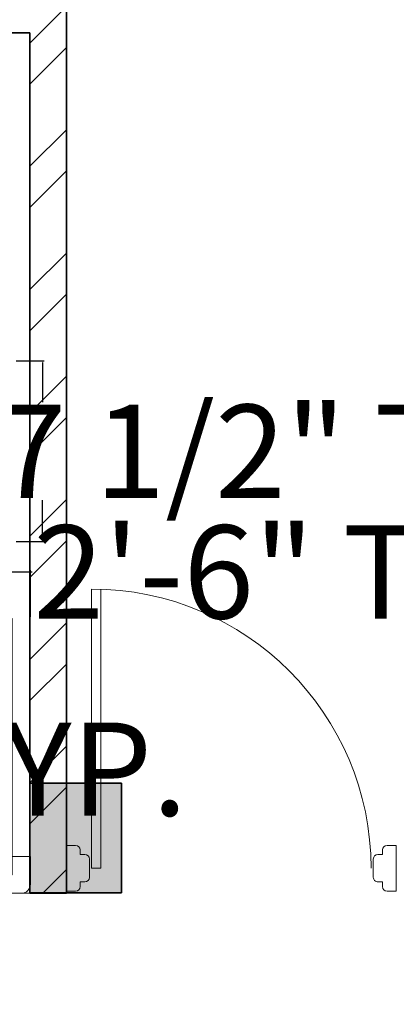
# Model space of a CAD drawing. Units: inches. Extents: x 1812 to 2791, y 2306 to 2959.
# Tile 6 of 8: x 2534 to 2575, y 2748 to 2856. Entities that reach past the tile are written whole.
import ezdxf

# ---------------------------------------------------------------- set-up
doc = ezdxf.new("R2010")
doc.units = ezdxf.units.IN
doc.layers.get('Defpoints').update_dxf_attribs({"lineweight": 50})
for name, color, linetype, lineweight in [('00 FURNITURE', 15, 'Continuous', 15), ('A-ANNO-DIMS', 2, 'Continuous', 18), ('A-COLS', 7, 'Continuous', 35), ('A-WALL-PATT', 8, 'Continuous', 13), ('A_FUR 1', 5, 'Continuous', 5), ('DOORS', 4, 'Continuous', 18), ('WALL', 7, 'Continuous', 35)]:
    doc.layers.add(name, color=color, linetype=linetype, lineweight=lineweight)
doc.styles.get("Standard").update_dxf_attribs({"font": 'arial.ttf'})
doc.dimstyles.get("Standard").update_dxf_attribs({"dimtxt": 10.18, "dimasz": 0.18, "dimexe": 0.18, "dimexo": 0.0625, "dimgap": 0.09, "dimtad": 0, "dimtih": 1, "dimtoh": 1, "dimdec": 0, "dimzin": 0, "dimdsep": 46, "dimlunit": 3, "dimtxsty": 'Standard', "dimcen": 0.09, "dimadec": 0, "dimazin": 0, "dimtfac": 1, "dimtdec": 0, "dimtofl": 0, "dimtmove": 0, "dimatfit": 3, "dimfxl": 1, "dimtolj": 1, "dimtzin": 0, "dimarcsym": 0})

# ---------------------------------------------------------------- blocks, each defined once
blk = doc.blocks.new('RGWTG')
at = {"layer": '00 FURNITURE'}
for p, q in [((578.2256807760662, 3473.505161377467), (577.3582404955016, 3475.007612015936)), ((578.3599178529946, 3473.582663189966), (577.4924775724302, 3475.085113828435)), ((578.2256807760662, 3473.582663189966), (577.3582404955016, 3472.080212551496)), ((578.3599178529946, 3473.505161377467), (577.4924775724302, 3472.002710738997)), ((578.2927993145303, 3473.621414096216), (580.0276798756596, 3473.621414096216)), ((578.2927993145303, 3473.466410471216), (580.0276798756596, 3473.466410471216)), ((521.9346502956948, 3464.582663189967), (509.0294035436774, 3451.677416437858)), ((509.0294035436774, 3422.632763190932), (509.0294035436774, 3463.682663189967)), ((509.9294035436774, 3464.582663189967), (566.4044035436774, 3464.582663189967)), ((557.5308429759127, 3463.839125240039), (557.5308429759127, 3464.490869196072)), ((557.5308429759127, 3464.490869196072), (566.4044035436774, 3464.490869196072)), ((558.2031535212662, 3464.490869196072), (558.2031535212662, 3435.82153971761)), ((559.5700285224608, 3464.490869196072), (559.5700285224608, 3437.251588151807)), ((560.936903521612, 3464.490869196072), (560.936903521612, 3438.58287176399)), ((562.3037785229637, 3464.490869196072), (562.3037785229637, 3439.825055824144)), ((563.670653522115, 3464.490869196072), (563.670653522115, 3440.98605097839)), ((565.0375285212663, 3464.490869196072), (565.0375285212663, 3442.08478108928)), ((566.4044035436774, 3464.582663189967), (580.984403544526, 3464.582663189967)), ((566.4044035436774, 3464.490869196072), (566.4044035436774, 3442.08478108928)), ((566.4044035436774, 3464.490869196072), (566.4044035436774, 3463.839125240039)), ((580.984403544526, 3464.582663189967), (580.984403544526, 3416.724846580601)), ((558.2031535212662, 3426.479299948917), (558.2031535212662, 3425.039797466598)), ((509.0294035436774, 3400.682663189967), (509.0294035436774, 3422.632763190932)), ((580.984403544526, 3416.724846580601), (580.984403544526, 3400.682663189967)), ((558.2031535212662, 3416.13290811762), (558.2031535212662, 3399.94638799492)), ((559.5700285224608, 3414.751712508814), (559.5700285224608, 3399.94638799492)), ((560.936903521612, 3413.388814481056), (560.936903521612, 3399.94638799492)), ((562.3037785229637, 3412.043853859778), (562.3037785229637, 3399.94638799492)), ((563.670653522115, 3410.716484398092), (563.670653522115, 3399.94638799492)), ((557.5308429759127, 3399.94638799492), (557.5308429759127, 3400.5981319509)), ((566.4044035436774, 3400.5981319509), (566.4044035436774, 3399.94638799492)), ((580.0844035445261, 3399.782663189967), (509.9294035436774, 3399.782663189967)), ((566.4044035436774, 3399.94638799492), (557.5308429759127, 3399.94638799492)), ((578.2256807760662, 3390.782663189968), (577.3582404955016, 3392.285113828438)), ((578.3599178529946, 3390.860165002467), (577.4924775724302, 3392.362615640937)), ((578.2256807760662, 3390.860165002467), (577.3582404955016, 3389.357714363998)), ((578.3599178529946, 3390.782663189968), (577.4924775724302, 3389.280212551498)), ((578.2927993145303, 3390.898915908717), (580.0276798756596, 3390.898915908717)), ((578.2927993145303, 3390.743912283717), (580.0276798756596, 3390.743912283717))]:
    blk.add_line(p, q, dxfattribs=at)
for points in [[(568.4294035436774, 3465.482663189967), (584.6294035436774, 3465.482663189967), (584.6294035436774, 3481.682663189967), (568.4294035436774, 3481.682663189967)], [(569.3294035436775, 3466.382663189967), (583.7294035436774, 3466.382663189967), (583.7294035436774, 3480.782663189966), (569.3294035436775, 3480.782663189966)], [(580.984403544526, 3399.782663189967), (584.6294035436774, 3399.782663189967), (584.6294035436774, 3464.582663189967), (580.984403544526, 3464.582663189967)], [(568.4294035436774, 3398.882663189967), (584.6294035436774, 3398.882663189967), (584.6294035436774, 3382.682663189966), (568.4294035436774, 3382.682663189966)], [(569.3294035436775, 3397.982663189967), (583.7294035436774, 3397.982663189967), (583.7294035436774, 3383.582663189967), (569.3294035436775, 3383.582663189967)]]:
    blk.add_lwpolyline(points, close=True, dxfattribs=at)
for points in [[(566.5249235009207, 3464.490869196072), (557.5308429759127, 3464.490869196072), (557.5308429759127, 3435.078372253239)], [(557.5308429759127, 3427.211042130029), (557.5308429759127, 3424.296630002226)], [(557.5308429759127, 3416.819089319545), (557.5308429759127, 3399.94638799492), (566.4044035436774, 3399.94638799492), (566.4044035436774, 3409.944208183064)]]:
    blk.add_lwpolyline(points, dxfattribs=at)
for centre, radius in [((578.2927993145303, 3473.543912283716), 3.969936732874747), ((578.2927993145303, 3473.543912283716), 3.628217982874746), ((578.2927993145303, 3473.543912283716), 1.736610806232817), ((578.2927993145303, 3473.543912283716), 1.556519175947022), ((578.2927993145303, 3390.821414096218), 3.969936732874747), ((578.2927993145303, 3390.821414096218), 3.628217982874746), ((578.2927993145303, 3390.821414096218), 1.736610806232817), ((578.2927993145303, 3390.821414096218), 1.556519175947022)]:
    blk.add_circle(centre, radius, dxfattribs=at)
for centre, radius, start, end in [((509.9294035436774, 3463.682663189967), 0.9, 90, 180), ((529.6454688338926, 3456.881544112086), 10.89788775774147, 135.036058935316, 191.9277514991085), ((290.5601735268501, 3490.521662704408), 268.3007568988695, 342.2213792030555, 354.2924942374134), ((516.7305226215815, 3443.966597899809), 10.89788775767012, 78.0722485009183, 134.9639410650166), ((566.0453802145915, 3440.566314355121), 1.822500000001211, 44.99999999963665, 135.0000000003634), ((533.5831293340844, 3399.312580336717), 54.3212999511223, 37.93095780394859, 52.06904219657574), ((598.1486039723109, 3399.008979125588), 54.3212999511223, 127.9309578034242, 142.0690421960514), ((574.836863352121, 3431.774831218586), 1.822500000001211, 315.0000000003633, 44.99999999963665), ((556.5912687458695, 3431.112202887551), 1.822500000001211, 135.0000000003634, 224.9999999996366), ((566.0453802145915, 3429.784572104108), 1.822500000001211, 44.99999999963665, 135.0000000003634), ((533.5831293340844, 3388.530838085705), 54.3212999511223, 37.93095780394859, 52.06904219657574), ((598.1486039723109, 3388.22723688411), 54.3212999511223, 127.9309578034242, 142.0690421960514), ((533.2795281258368, 3463.878054972429), 54.3212999511223, 316.3199934856352, 322.0690421960514), ((597.8663488484293, 3463.595799850381), 54.3212999511223, 217.9309578039486, 224.1410097173259), ((574.836863352121, 3420.993088967574), 1.822500000001211, 315.0000000003633, 44.99999999963665), ((556.5912687458695, 3420.330460636539), 1.822500000001211, 135.0000000003634, 224.9999999996366), ((533.2795281258368, 3453.096312729537), 54.3212999511223, 307.9309578034243, 322.0690421960514), ((765.333036254045, 3619.748261904361), 290.4513739299737, 223.6068611219581, 226.2326326311176), ((565.4405781886671, 3411.054704570479), 1.470429037080631, 225.9674007983825, 326.8336929335584), ((545.0195012894181, 3395.287888507475), 13.35047895143779, 20.42241827524089, 85.58252621369252), ((509.9294035436774, 3400.682663189967), 0.9, 180, 270), ((580.0844035445261, 3400.682663189967), 0.9, 270, 0)]:
    blk.add_arc(centre, radius, start, end, dxfattribs=at)
blk = doc.blocks.new('DDD')
at = {"layer": '00 FURNITURE'}
for p, q in [((-12579.77346126611, -15859.52901419652), (-12579.77346126608, -15829.04541204713)), ((-12578.77346126611, -15859.52901419657), (-12578.77346126608, -15829.02901419657)), ((-12612.02346126613, -15857.02901419646), (-12612.02346126613, -15862.02901419646)), ((-12611.02346126613, -15857.02901419646), (-12612.02346126613, -15857.02901419646)), ((-12577.02346126611, -15857.02901419657), (-12576.02346126611, -15857.02901419652)), ((-12576.02346126611, -15857.02901419652), (-12576.02346126611, -15862.02901419652)), ((-12610.52346126612, -15858.02901419646), (-12610.52346126612, -15857.52901419646)), ((-12577.52346126611, -15858.02901419658), (-12577.52346126611, -15857.52901419657)), ((-12578.77346126611, -15859.52901419657), (-12579.77346126611, -15859.52901419652)), ((-12610.52346126612, -15861.52901419646), (-12610.52346126612, -15861.02901419646)), ((-12577.52346126611, -15861.52901419657), (-12577.52346126611, -15861.02901419657)), ((-12612.02346126613, -15862.02901419646), (-12611.02346126613, -15862.02901419646)), ((-12576.02346126611, -15862.02901419652), (-12577.02346126611, -15862.02901419657))]:
    blk.add_line(p, q, dxfattribs=at)
for points in [[(-12610.52346126612, -15861.02901419646), (-12610.02346126613, -15861.02901419646, 0.4142135623730951), (-12609.52346126612, -15860.52901419646), (-12609.52346126612, -15858.52901419646, 0.4142135623730951), (-12610.02346126613, -15858.02901419646), (-12610.52346126612, -15858.02901419646)], [(-12577.52346126611, -15861.02901419657), (-12578.02346126611, -15861.02901419657, -0.4142135623730951), (-12578.52346126611, -15860.52901419657), (-12578.52346126611, -15858.52901419657, -0.4142135623730951), (-12578.02346126611, -15858.02901419658), (-12577.52346126611, -15858.02901419658)]]:
    blk.add_lwpolyline(points, format="xyb", dxfattribs=at)
for centre, radius, start, end in [((-12578.77346126613, -15859.52901419657), 30.49999999999949, 90, 180), ((-12611.02346126613, -15857.52901419646), 0.4999999999999916, 0, 90), ((-12577.02346126611, -15857.52901419657), 0.4999999999999916, 90, 180), ((-12611.02346126613, -15861.52901419646), 0.4999999999999916, 270, 0), ((-12577.02346126611, -15861.52901419657), 0.4999999999999916, 180, 270)]:
    blk.add_arc(centre, radius, start, end, dxfattribs=at)
blk = doc.blocks.new('ESTSET')
at = {"layer": 'A_FUR 1'}
for p, q in [((-10.44359699611232, 4.096573562603225), (-10.44359699611232, 32.09657356260323)), ((-8.44359699611232, 4.096573562603225), (-8.44359699611232, 32.09657356260323)), ((-36.44359699611232, 6.096573562603225), (-36.44359699611232, 3.096573562603225)), ((-34.44359699611232, 6.096573562603225), (-36.44359699611232, 6.096573562603225)), ((-34.44359699611232, 4.096573562603225), (-34.44359699611232, 6.096573562603225)), ((-34.44359699611232, 4.096573562603225), (-34.44359699611232, 6.096573562603225)), ((-8.44359699611232, 4.096573562603225), (-8.44359699611232, 6.096573562603225)), ((-8.44359699611232, 6.096573562603225), (-6.443596996112319, 6.096573562603225)), ((-8.44359699611232, 4.096573562603225), (-8.44359699611232, 6.096573562603225)), ((-6.443596996112319, 6.096573562603225), (-6.443596996112319, 3.096573562603225)), ((-32.44359699611232, 4.096573562603225), (-34.44359699611232, 4.096573562603225)), ((-32.44359699611232, 4.096573562603225), (-34.44359699611232, 4.096573562603225)), ((-32.44359699611232, 3.096573562603225), (-32.44359699611232, 4.096573562603225)), ((-10.44359699611232, 3.096573562603225), (-10.44359699611232, 4.096573562603225)), ((-10.44359699611232, 4.096573562603225), (-8.44359699611232, 4.096573562603225)), ((-10.44359699611232, 4.096573562603225), (-8.44359699611232, 4.096573562603225)), ((-6.443596996112319, 2.096573562601521), (-36.4435969961196, 2.09657356260334)), ((-35.44359699611232, 2.096573562603225), (-33.44359699611232, 2.096573562603225)), ((-7.443596996112319, 2.096573562603225), (-9.44359699611232, 2.096573562603225))]:
    blk.add_line(p, q, dxfattribs=at)
for points in [[(-21.44359699614506, 2.09657356260334), (-18.67227073841423, 2.09657356260334), (-18.67227073841423, 5.101808480258228), (-20.05793386727964, 5.101808480258228)], [(-20.05793386727964, 5.101808480258228), (-20.05793386727964, -0.9086613550515485)], [(-21.44359699614506, 2.09657356260334), (-21.44359699614506, -0.9086613550515485), (-20.05793386727964, -0.9086613550515485)]]:
    blk.add_lwpolyline(points, dxfattribs=at)
for centre, radius, start, end in [((-8.908777800232201, 6.457098594999479), 25.64369454261379, 88.96058819788949, 185.2816045955121), ((-35.44359699611232, 3.096573562603225), 1, 180, 270), ((-33.44359699611232, 3.096573562603225), 1, 270, 0), ((-9.44359699611232, 3.096573562603225), 1, 180, 270), ((-7.443596996112319, 3.096573562603225), 1, 270, 0)]:
    blk.add_arc(centre, radius, start, end, dxfattribs=at)
blk = doc.blocks.new('COL')
at = {"transparency": 33554687}
h = blk.add_hatch(color=256, dxfattribs=at)
h.dxf.hatch_style = 1
h.paths.add_polyline_path([(2424.397880689844, 2829.240948453883), (2424.397880689844, 2839.240948453883), (2412.397880689843, 2839.240948453883), (2412.397880689843, 2829.240948453883)])
for p, q in [((2412.397880689843, 2839.240948453883), (2424.397880689844, 2839.240948453883)), ((2412.397880689843, 2839.240948453883), (2412.397880689843, 2829.240948453882)), ((2424.397880689844, 2839.240948453883), (2424.397880689844, 2829.240948453883)), ((2412.397880689843, 2829.240948453883), (2424.397880689844, 2829.240948453883))]:
    blk.add_line(p, q)
blk = doc.blocks.new('*D58')
at = {"layer": 'A-ANNO-DIMS', "color": 0, "lineweight": -2, "transparency": 16777216}
for p, q in [((2533.666907414658, 2818.774380578327), (2536.746255119824, 2818.774380578327)), ((2536.566255119824, 2818.594380578328), (2536.566255119824, 2814.255156531551)), ((2536.566255119824, 2799.20872921056), (2536.566255119824, 2803.547953257336)), ((2533.666907414658, 2799.02872921056), (2536.746255119824, 2799.02872921056))]:
    blk.add_line(p, q, dxfattribs=at)
at = {"layer": 'A-ANNO-DIMS', "color": 0, "transparency": 16777216}
for points in [[(2536.536255119824, 2818.594380578328), (2536.596255119824, 2818.594380578328), (2536.566255119824, 2818.774380578327)], [(2536.536255119824, 2799.20872921056), (2536.596255119824, 2799.20872921056), (2536.566255119824, 2799.02872921056)]]:
    blk.add_solid(points, dxfattribs=at)
at = {"layer": 'Defpoints', "color": 0, "transparency": 16777216}
for p in [(2533.604407414657, 2818.774380578327), (2533.604407414657, 2799.02872921056), (2536.566255119824, 2799.02872921056)]:
    blk.add_point(p, dxfattribs=at)
at = {"layer": 'A-ANNO-DIMS', "color": 0, "transparency": 16777216, "insert": (2536.566255119824, 2808.901554894443), "char_height": 10.18, "attachment_point": 5}
blk.add_mtext('\\A1;BASIN 1\'-7 1/2" TYP.', dxfattribs=at)
blk = doc.blocks.new('*D60')
at = {"layer": 'A-ANNO-DIMS', "color": 0, "lineweight": -2, "transparency": 16777216}
for p, q in [((2505.177694196558, 2790.74953182163), (2500.089565400664, 2790.74953182163)), ((2500.269565400663, 2790.56953182163), (2500.269565400663, 2779.537842838497)), ((2500.269565400663, 2757.792006515665), (2500.269565400663, 2768.823695498797)), ((2505.177694196558, 2757.612006515665), (2500.089565400664, 2757.612006515665))]:
    blk.add_line(p, q, dxfattribs=at)
at = {"layer": 'A-ANNO-DIMS', "color": 0, "transparency": 16777216}
for points in [[(2500.239565400664, 2790.56953182163), (2500.299565400664, 2790.56953182163), (2500.269565400663, 2790.74953182163)], [(2500.239565400664, 2757.792006515665), (2500.299565400664, 2757.792006515665), (2500.269565400663, 2757.612006515665)]]:
    blk.add_solid(points, dxfattribs=at)
at = {"layer": 'Defpoints', "color": 0, "transparency": 16777216}
for p in [(2500.269565400663, 2790.74953182163), (2505.240194196558, 2790.74953182163), (2505.240194196558, 2757.612006515665)]:
    blk.add_point(p, dxfattribs=at)
at = {"layer": 'A-ANNO-DIMS', "color": 0, "transparency": 16777216, "insert": (2500.269565400663, 2774.180769168646), "char_height": 10.18, "attachment_point": 5}
blk.add_mtext('\\A1;DOOR 2\'-9" TYP.', dxfattribs=at)
blk = doc.blocks.new('*D61')
at = {"layer": 'A-ANNO-DIMS', "color": 0, "lineweight": -2, "transparency": 16777216}
for p, q in [((2505.240194196556, 2790.812031821629), (2505.240194196556, 2795.900160617524)), ((2505.420194196557, 2795.720160617524), (2535.060194196564, 2795.720160617524)), ((2535.240194196564, 2790.812031821629), (2535.240194196564, 2795.900160617524)), ((2535.240194196564, 2795.720160617524), (2535.420194196563, 2795.720160617524))]:
    blk.add_line(p, q, dxfattribs=at)
at = {"layer": 'A-ANNO-DIMS', "color": 0, "transparency": 16777216}
for points in [[(2505.420194196557, 2795.750160617524), (2505.420194196557, 2795.690160617523), (2505.240194196556, 2795.720160617524)], [(2535.060194196564, 2795.750160617524), (2535.060194196564, 2795.690160617523), (2535.240194196564, 2795.720160617524)]]:
    blk.add_solid(points, dxfattribs=at)
at = {"layer": 'Defpoints', "color": 0, "transparency": 16777216}
for p in [(2535.240194196564, 2795.720160617524), (2505.240194196556, 2790.749531821629), (2535.240194196564, 2790.749531821629)]:
    blk.add_point(p, dxfattribs=at)
at = {"layer": 'A-ANNO-DIMS', "color": 0, "transparency": 16777216, "insert": (2566.623079599019, 2795.720160617524), "char_height": 10.18, "attachment_point": 5}
blk.add_mtext('\\A1;2\'-6" TYP.', dxfattribs=at)
blk = doc.blocks.new('*D64')
at = {"layer": 'A-ANNO-DIMS', "color": 0, "lineweight": -2, "transparency": 16777216}
for p, q in [((2499.736887761388, 2721.901978502181), (2499.736887761388, 2724.667753417118)), ((2517.392053860968, 2721.901978502181), (2517.392053860968, 2724.667753417118)), ((2499.916887761388, 2724.487753417118), (2517.212053860968, 2724.487753417118)), ((2517.392053860968, 2724.487753417118), (2517.572053860968, 2724.487753417118))]:
    blk.add_line(p, q, dxfattribs=at)
at = {"layer": 'A-ANNO-DIMS', "color": 0, "transparency": 16777216}
for points in [[(2499.916887761388, 2724.517753417118), (2499.916887761388, 2724.457753417118), (2499.736887761388, 2724.487753417118)], [(2517.212053860968, 2724.517753417118), (2517.212053860968, 2724.457753417118), (2517.392053860968, 2724.487753417118)]]:
    blk.add_solid(points, dxfattribs=at)
at = {"layer": 'Defpoints', "color": 0, "transparency": 16777216}
for p in [(2517.392053860968, 2724.487753417118), (2499.736887761388, 2721.839478502181), (2517.392053860968, 2721.839478502181)]:
    blk.add_point(p, dxfattribs=at)
at = {"layer": 'A-ANNO-DIMS', "color": 0, "transparency": 16777216, "insert": (2601.369291241595, 2724.487753417118), "char_height": 10.18, "attachment_point": 5}
blk.add_mtext('\\A1;END CHAIR 1\'-5 1/2" TYP.', dxfattribs=at)

msp = doc.modelspace()

# ---------------------------------------------------------------- hatches: boundary and pattern name
at = {"layer": 'A-WALL-PATT'}
h = msp.add_hatch(dxfattribs=at)
h.set_pattern_fill('ANSI32', color=256)
h.set_pattern_definition([(45, (563.8057507655523, 20.01067828916757), (-6.735192090801865, 6.735192090801866), []), (45, (568.2958807655523, 20.01067828916757), (-6.735192090801865, 6.735192090801866), [])])
h.paths.add_polyline_path([(2694.192292649419, 2437.613622010101), (2683.499516441466, 2437.6136220101), (2683.499516441466, 2788.569354872347), (2685.192292649419, 2788.569354872347), (2685.192292649419, 2821.63505754476), (2685.125860943268, 2869.374403893766), (2685.125860943268, 2821.63505754476), (2694.192292649419, 2821.63505754476)])
h.paths.add_polyline_path([(2587.192292649419, 2446.613622010096), (2463.19229264942, 2446.613622010089), (2463.19229264942, 2473.613622010101), (2515.608214234135, 2473.613622010101), (2515.608214234135, 2477.6136220101), (2463.19229264942, 2477.6136220101), (2463.19229264942, 2610.6136220101), (2523.737487215154, 2610.613622010101), (2523.737487215154, 2614.613622010101), (2463.19229264942, 2614.6136220101), (2463.19229264942, 2654.536135698824), (2454.192292649419, 2654.536135698824), (2454.192292649419, 2437.613622010101), (2587.192292649419, 2437.613622010101)])
h.paths.add_polyline_path([(2683.499516441466, 2446.6136220101), (2676.19229264942, 2446.6136220101), (2676.192292649419, 2437.6136220101), (2683.499516441466, 2437.613622010101)])
h.paths.add_polyline_path([(2463.192292649419, 2760.6136220101), (2505.192292649419, 2760.6136220101), (2505.192292649419, 2764.6136220101), (2463.192292649419, 2764.6136220101), (2463.192292649419, 2792.952050683902), (2454.192292649419, 2792.952050683902), (2454.192292649419, 2702.536135698824), (2463.016486285651, 2702.536135698824), (2463.016486285651, 2702.649195550402)])
h.paths.add_polyline_path([(2539.192292649419, 2858.613622010101), (2463.192292649419, 2858.6136220101), (2463.192292649419, 2876.345134993912), (2454.192292649419, 2876.345134993912), (2454.19229264942, 2816.957881357627), (2463.192292649419, 2816.957881357627), (2463.192292649419, 2854.6136220101), (2535.192292649419, 2854.613622010101), (2535.192292649419, 2760.6136220101), (2539.192292649419, 2760.6136220101)])
h.paths.add_polyline_path([(2683.499516441466, 2917.613622010101), (2454.192292649419, 2917.613622010101), (2454.192292649419, 2900.372408669677), (2463.192292649419, 2900.372408669677), (2463.192292649419, 2908.6136220101), (2683.499516441466, 2908.613622010101)])
h.paths.add_polyline_path([(2694.192292649419, 2917.613622010101), (2683.499516441466, 2917.613622010101), (2683.499516441466, 2908.613622010101), (2685.192292649419, 2908.613622010101), (2685.192292649419, 2869.63505754476), (2694.192292649419, 2869.63505754476)])

# ---------------------------------------------------------------- linework, layer by layer
at = {"layer": 'WALL'}
for p, q in [((2539.192292649419, 2760.6136220101), (2539.192292649419, 2858.6136220101)), ((2463.19229264942, 2854.6136220101), (2535.192292649419, 2854.613622010101)), ((2535.192292649419, 2760.6136220101), (2535.192292649419, 2854.613622010101)), ((2535.19229264942, 2760.6136220101), (2539.192292649419, 2760.6136220101))]:
    msp.add_line(p, q, dxfattribs=at)

# ---------------------------------------------------------------- block references
at = {"layer": '00 FURNITURE', "xscale": -1, "rotation": 270}
msp.add_blockref('RGWTG', (-808.2006863094902, 2322.539075156897), dxfattribs=at)
at = {"layer": 'A-COLS', "rotation": 270}
msp.add_blockref('COL', (-294.053850132259, 5185.043230545718), dxfattribs=at)
at = {"layer": 'DOORS', "xscale": -1}
msp.add_blockref('DDD', (-10036.84713077235, 18622.87667993446), dxfattribs=at)
at = {"layer": 'DOORS'}
msp.add_blockref('ESTSET', (2541.683791192676, 2758.520667870716), dxfattribs=at)

# ---------------------------------------------------------------- dimensions: what is measured, and where the dimension line sits
at = {"layer": 'A-ANNO-DIMS'}
for base, p1, p2, angle, text, picture, middle in [((2536.566255119824, 2799.02872921056), (2533.604407414657, 2818.774380578327), (2533.604407414657, 2799.028729210559), 270, 'BASIN <> TYP.', '*D58', (2536.566255119824, 2808.901554894443)), ((2500.269565400663, 2790.74953182163), (2505.240194196556, 2757.612006515664), (2505.240194196556, 2790.749531821629), 90, 'DOOR <> TYP.', '*D60', (2500.269565400663, 2774.180769168646))]:
    dim = msp.add_linear_dim(base=base, p1=p1, p2=p2, angle=angle, text=text, dimstyle='Standard', override={"dimdec": 1, "dimlfac": 1, "dimrnd": 0, "dimzin": 1, "dimdsep": 46, "dimlunit": 4, "dimfrac": 2}, dxfattribs=at)
    dim.commit()
    dim.dimension.update_dxf_attribs({"geometry": picture, "text_midpoint": middle})
for base, p1, p2, text, picture, middle in [((2535.240194196564, 2795.720160617524), (2505.240194196556, 2790.749531821629), (2535.240194196564, 2790.749531821629), '<> TYP.', '*D61', (2566.623079599019, 2795.720160617524)), ((2517.392053860968, 2724.487753417118), (2499.736887761388, 2721.839478502181), (2517.392053860968, 2721.839478502181), 'END CHAIR <> TYP.', '*D64', (2601.369291241595, 2724.487753417118))]:
    dim = msp.add_linear_dim(base=base, p1=p1, p2=p2, text=text, dimstyle='Standard', override={"dimdec": 1, "dimlfac": 1, "dimrnd": 0, "dimzin": 1, "dimdsep": 46, "dimlunit": 4, "dimfrac": 2}, dxfattribs=at)
    dim.commit()
    dim.dimension.update_dxf_attribs({"geometry": picture, "text_midpoint": middle})

doc.saveas('drawing.dxf')
